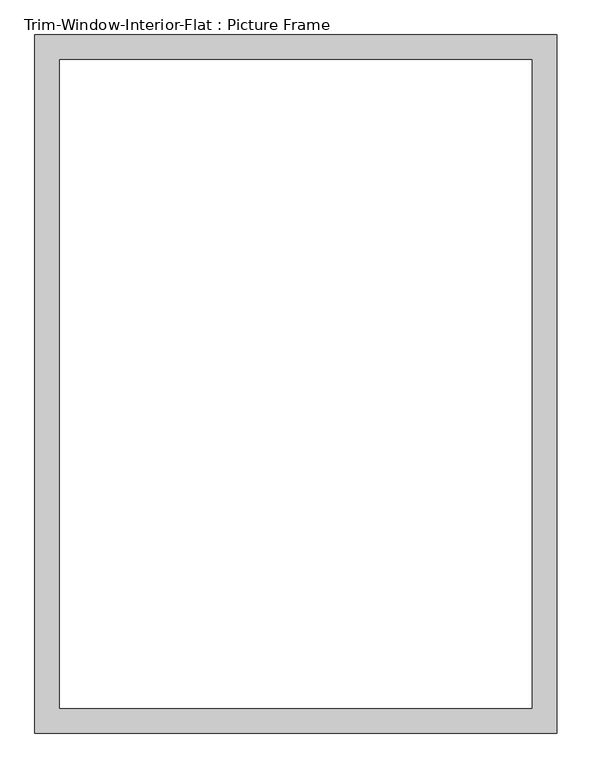
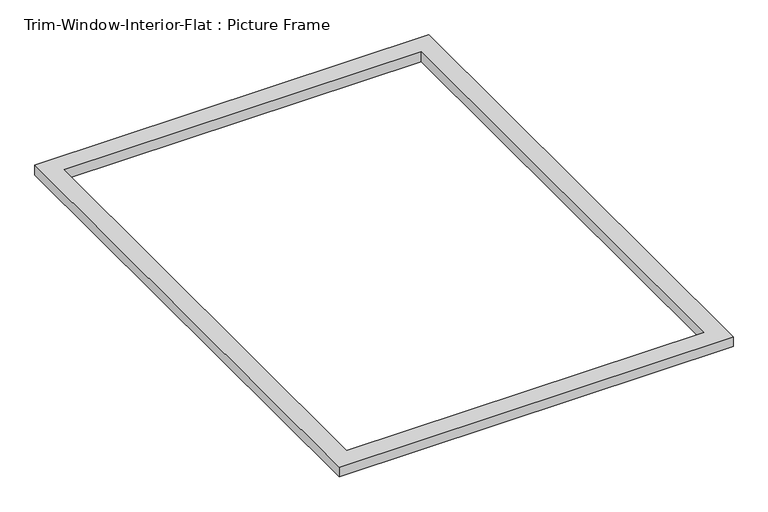
"""IFC4 building model written with IfcOpenShell, lengths in millimetres: proxy geometry, Trim-Window-Interior-Flat : Picture Frame."""

from ifc_helpers import new_model, si_unit, origin, origin_with_axes, place, context, project, spatial, polyline, outline, extrude, source, transform, mapped, element, save


def trim_window_interior_flat_picture_frame_d06e6fc7(model_context):
    return source(origin(), model_context, "Body", "SweptSolid", [
        extrude(outline(polyline([(603.25, 44.45), (603.25, -1568.45), (-603.25, -1568.45), (-603.25, 44.45), (603.25, 44.45)]), holes=[polyline([(546.1, -12.7), (-546.1, -12.7), (-546.1, -1511.3), (546.1, -1511.3), (546.1, -12.7)])]), origin_with_axes(), (0.0, 0.0, 1.0), 31.75),
    ])


if __name__ == "__main__":
    model = new_model("IFC4")
    model_context = context("Model", 3, world=origin())
    ifc_project = project(units=[si_unit("LENGTHUNIT", "METRE", prefix="MILLI")], contexts=[model_context])
    site = spatial("IfcSite", under=ifc_project)
    building = spatial("IfcBuilding", under=site)
    placement = place(None, origin())
    trim_window_interior_flat_picture_frame_shape = trim_window_interior_flat_picture_frame_d06e6fc7(model_context)
    element("IfcBuildingElementProxy", 1, Name="Trim-Window-Interior-Flat : Picture Frame", ObjectType="Trim-Window-Interior-Flat : Picture Frame", at=placement, inside=building, context=model_context, shape_type="MappedRepresentation", body=[
        mapped(trim_window_interior_flat_picture_frame_shape, transform((0.0, 0.0, 0.0), x_axis=(1.0, 0.0, 0.0), y_axis=(0.0, 1.0, 0.0), z_axis=(0.0, 0.0, 1.0))),
    ])
    save(model, "model.ifc")

# Revit data of these elements
# Type "Trim-Window-Interior-Flat : Picture Frame"
#   Trim Thickness_Picture Frame = 0' - 1 1/4"
#   Trim Width = 0' - 2 1/4"
#   Trim Thickness_with Sill = 0' - 0 3/4"
#   Sill Thickness = 0' - 1 1/4"
#   Opening Width [instance default] = 2' - 0"
#   Opening Height [instance default] = 3' - 0"
#   Default Elevation = 4' - 0"
#   Sill = no
#   Picture Frame = yes
#   Trim Material [instance default] = none
# Element 1 (IfcBuildingElementProxy, "Trim-Window-Interior-Flat : Picture Frame")
#   Opening Width = 3' - 8"
#   Opening Height = 5' - 0"
#   Trim Material = Wood - Stained
#   Materials on its faces: "Wood - Stained"
# Materials
#   "Wood - Stained": class "Wood", colour RGB 224 178 126, transparency 0, Cost = 0
